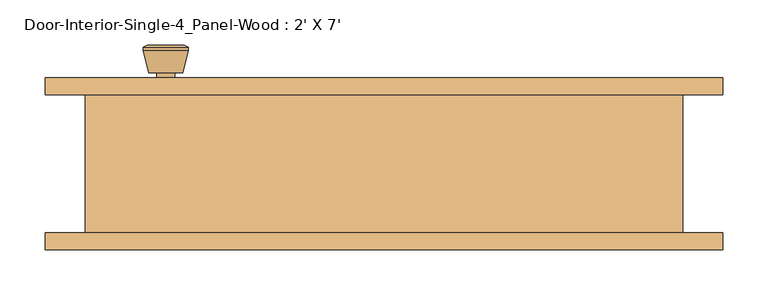
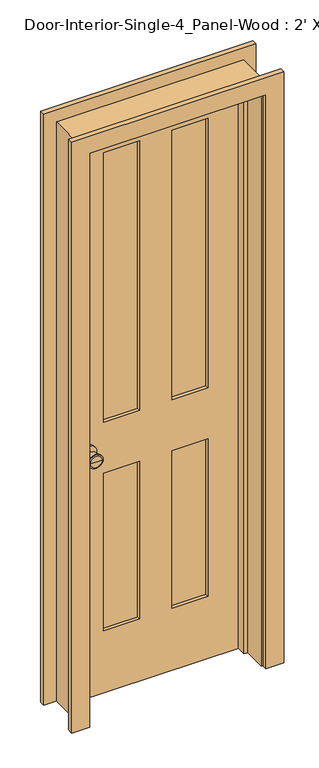
"""IFC4 building model written with IfcOpenShell, lengths in millimetres: door geometry, Door-Interior-Single-4_Panel-Wood : 2' X 7'."""

from ifc_helpers import new_model, si_unit, point, frame, frame_2d, origin, place, context, project, spatial, polyline, circle_curve, trimmed, segment, composite_curve, outline, extrude, faceted_brep, source, transform, mapped, element, save
from ifc_brep_helpers import plane_surface, cylinder_surface, revolved_surface, advanced_brep


def door_interior_single_4_panel_wood_2_x_7_099afc9e(model_context):
    return source(origin(), model_context, "Body", "SolidModel", [
        advanced_brep(
        [(-241.3, 32.1, 914.4), (-231.3, 32.1, 914.4), (-251.3, 32.1, 914.4), (-220.8241324, -16.9, 914.4), (-241.3, -16.9, 914.4), (-261.7758676, -16.9, 914.4), (-216.3, -15.0721319, 914.4), (-266.3, -15.0721319, 914.4), (-216.3, -11.6084537, 914.4), (-266.3, -11.6084537, 914.4), (-222.663764, 13.1, 914.4), (-259.936236, 13.1, 914.4), (-231.3, 13.1, 914.4), (-251.3, 13.1, 914.4)],
        [
            (0, 1),
            (1, 2, circle_curve(frame((-241.3, 32.1, 914.4), z_axis=(0.0, 1.0, 0.0), x_axis=(-1.0, 0.0, 0.0)), 10.0)),
            (2, 0),
            (2, 1, circle_curve(frame((-241.3, 32.1, 914.4), z_axis=(0.0, 1.0, 0.0), x_axis=(-1.0, 0.0, 0.0)), 10.0)),
            (3, 4),
            (4, 5),
            (5, 3, circle_curve(frame((-241.3, -16.9, 914.4), z_axis=(0.0, -1.0, 0.0), x_axis=(-1.0, 0.0, 0.0)), 20.4758676)),
            (3, 5, circle_curve(frame((-241.3, -16.9, 914.4), z_axis=(0.0, -1.0, 0.0), x_axis=(-1.0, 0.0, 0.0)), 20.4758676)),
            (6, 3),
            (5, 7),
            (7, 6, circle_curve(frame((-241.3, -15.0721319, 914.4), z_axis=(0.0, -1.0, 0.0), x_axis=(-1.0, 0.0, 0.0)), 25.0)),
            (6, 7, circle_curve(frame((-241.3, -15.0721319, 914.4), z_axis=(0.0, -1.0, 0.0), x_axis=(-1.0, 0.0, 0.0)), 25.0)),
            (8, 6),
            (7, 9),
            (9, 8, circle_curve(frame((-241.3, -11.6084537, 914.4), z_axis=(0.0, -1.0, 0.0), x_axis=(-1.0, 0.0, 0.0)), 25.0)),
            (8, 9, circle_curve(frame((-241.3, -11.6084537, 914.4), z_axis=(0.0, -1.0, 0.0), x_axis=(-1.0, 0.0, 0.0)), 25.0)),
            (10, 8),
            (9, 11),
            (11, 10, circle_curve(frame((-241.3, 13.1, 914.4), z_axis=(0.0, -1.0, 0.0), x_axis=(-1.0, 0.0, 0.0)), 18.636236)),
            (10, 11, circle_curve(frame((-241.3, 13.1, 914.4), z_axis=(0.0, -1.0, 0.0), x_axis=(-1.0, 0.0, 0.0)), 18.636236)),
            (12, 10),
            (11, 13),
            (13, 12, circle_curve(frame((-241.3, 13.1, 914.4), z_axis=(0.0, -1.0, 0.0), x_axis=(-1.0, 0.0, 0.0)), 10.0)),
            (12, 13, circle_curve(frame((-241.3, 13.1, 914.4), z_axis=(0.0, -1.0, 0.0), x_axis=(-1.0, 0.0, 0.0)), 10.0)),
            (1, 12),
            (13, 2),
        ],
        [
            plane_surface(frame((-241.3, 32.1, 914.4), z_axis=(0.0, 1.0, 0.0), x_axis=(-1.0, 0.0, 0.0))),
            plane_surface(frame((-241.3, -16.9, 914.4), z_axis=(0.0, -1.0, 0.0), x_axis=(-1.0, 0.0, 0.0))),
            revolved_surface(polyline([(-261.7758676, -16.9, 914.4), (-266.3, -15.0721319, 914.4)]), (-241.3, 32.1, 914.4), (0.0, 1.0, 0.0)),
            cylinder_surface(frame((-241.3, 32.1, 914.4), z_axis=(0.0, 1.0, 0.0), x_axis=(-1.0, 0.0, 0.0)), 25.0),
            revolved_surface(polyline([(-266.3, -11.6084537, 914.4), (-259.936236, 13.1, 914.4)]), (-241.3, 32.1, 914.4), (0.0, 1.0, 0.0)),
            plane_surface(frame((-241.3, 13.1, 914.4), z_axis=(0.0, 1.0, 0.0), x_axis=(-1.0, 0.0, 0.0))),
            cylinder_surface(frame((-241.3, 32.1, 914.4), z_axis=(0.0, 1.0, 0.0), x_axis=(-1.0, 0.0, 0.0)), 10.0),
        ],
        [
            (0, [[1, 2, 3]]),
            (0, [[-3, 4, -1]]),
            (1, [[5, 6, 7]]),
            (1, [[-6, -5, 8]]),
            (2, [[9, -7, 10, 11]]),
            (2, [[-10, -8, -9, 12]]),
            (3, [[13, -11, 14, 15]]),
            (3, [[-14, -12, -13, 16]]),
            (4, [[17, -15, 18, 19]]),
            (4, [[-18, -16, -17, 20]]),
            (5, [[21, -19, 22, 23]]),
            (5, [[-22, -20, -21, 24]]),
            (6, [[25, -23, 26, -2]]),
            (6, [[-26, -24, -25, -4]]),
        ],
    ),
        extrude(outline(composite_curve([segment(trimmed(circle_curve(frame_2d((914.4, -241.3)), 30.0), [point((914.4, -271.3))], [point((914.4, -211.3))], False, "CARTESIAN"), True, "CONTINUOUS"), segment(trimmed(circle_curve(frame_2d((914.4, -241.3)), 30.0), [point((914.4, -211.3))], [point((914.4, -271.3))], False, "CARTESIAN"), True, "CONTINUOUS")], self_intersect=False)), frame((0.0, 32.1, 0.0), z_axis=(0.0, 1.0, 0.0), x_axis=(0.0, 0.0, 1.0)), (0.0, 0.0, 1.0), 6.0),
        advanced_brep(
        [(-241.3, 79.025, 914.4), (-251.3, 79.025, 914.4), (-231.3, 79.025, 914.4), (-220.8241324, 128.025, 914.4), (-261.7758676, 128.025, 914.4), (-241.3, 128.025, 914.4), (-216.3, 126.1971319, 914.4), (-266.3, 126.1971319, 914.4), (-216.3, 122.7334537, 914.4), (-266.3, 122.7334537, 914.4), (-222.663764, 98.025, 914.4), (-259.936236, 98.025, 914.4), (-231.3, 98.025, 914.4), (-251.3, 98.025, 914.4)],
        [
            (0, 1),
            (1, 2, circle_curve(frame((-241.3, 79.025, 914.4), z_axis=(0.0, -1.0, 0.0), x_axis=(-1.0, 0.0, 0.0)), 10.0)),
            (2, 0),
            (2, 1, circle_curve(frame((-241.3, 79.025, 914.4), z_axis=(0.0, -1.0, 0.0), x_axis=(-1.0, 0.0, 0.0)), 10.0)),
            (3, 4, circle_curve(frame((-241.3, 128.025, 914.4), z_axis=(0.0, 1.0, 0.0), x_axis=(-1.0, 0.0, 0.0)), 20.4758676)),
            (4, 5),
            (5, 3),
            (4, 3, circle_curve(frame((-241.3, 128.025, 914.4), z_axis=(0.0, 1.0, 0.0), x_axis=(-1.0, 0.0, 0.0)), 20.4758676)),
            (6, 7, circle_curve(frame((-241.3, 126.1971319, 914.4), z_axis=(0.0, 1.0, 0.0), x_axis=(-1.0, 0.0, 0.0)), 25.0)),
            (7, 4),
            (3, 6),
            (7, 6, circle_curve(frame((-241.3, 126.1971319, 914.4), z_axis=(0.0, 1.0, 0.0), x_axis=(-1.0, 0.0, 0.0)), 25.0)),
            (8, 9, circle_curve(frame((-241.3, 122.7334537, 914.4), z_axis=(0.0, 1.0, 0.0), x_axis=(-1.0, 0.0, 0.0)), 25.0)),
            (9, 7),
            (6, 8),
            (9, 8, circle_curve(frame((-241.3, 122.7334537, 914.4), z_axis=(0.0, 1.0, 0.0), x_axis=(-1.0, 0.0, 0.0)), 25.0)),
            (10, 11, circle_curve(frame((-241.3, 98.025, 914.4), z_axis=(0.0, 1.0, 0.0), x_axis=(-1.0, 0.0, 0.0)), 18.636236)),
            (11, 9),
            (8, 10),
            (11, 10, circle_curve(frame((-241.3, 98.025, 914.4), z_axis=(0.0, 1.0, 0.0), x_axis=(-1.0, 0.0, 0.0)), 18.636236)),
            (12, 13, circle_curve(frame((-241.3, 98.025, 914.4), z_axis=(0.0, 1.0, 0.0), x_axis=(-1.0, 0.0, 0.0)), 10.0)),
            (13, 11),
            (10, 12),
            (13, 12, circle_curve(frame((-241.3, 98.025, 914.4), z_axis=(0.0, 1.0, 0.0), x_axis=(-1.0, 0.0, 0.0)), 10.0)),
            (1, 13),
            (12, 2),
        ],
        [
            plane_surface(frame((-241.3, 79.025, 914.4), z_axis=(0.0, -1.0, 0.0), x_axis=(-1.0, 0.0, 0.0))),
            plane_surface(frame((-241.3, 128.025, 914.4), z_axis=(0.0, 1.0, 0.0), x_axis=(-1.0, 0.0, 0.0))),
            revolved_surface(polyline([(-261.7758676, 128.025, 914.4), (-266.3, 126.1971319, 914.4)]), (-241.3, 79.025, 914.4), (0.0, -1.0, 0.0)),
            cylinder_surface(frame((-241.3, 79.025, 914.4), z_axis=(0.0, -1.0, 0.0), x_axis=(-1.0, 0.0, 0.0)), 25.0),
            revolved_surface(polyline([(-266.3, 122.7334537, 914.4), (-259.936236, 98.025, 914.4)]), (-241.3, 79.025, 914.4), (0.0, -1.0, 0.0)),
            plane_surface(frame((-241.3, 98.025, 914.4), z_axis=(0.0, -1.0, 0.0), x_axis=(-1.0, 0.0, 0.0))),
            cylinder_surface(frame((-241.3, 79.025, 914.4), z_axis=(0.0, -1.0, 0.0), x_axis=(-1.0, 0.0, 0.0)), 10.0),
        ],
        [
            (0, [[1, 2, 3]]),
            (0, [[-3, 4, -1]]),
            (1, [[5, 6, 7]]),
            (1, [[8, -7, -6]]),
            (2, [[9, 10, -5, 11]]),
            (2, [[12, -11, -8, -10]]),
            (3, [[13, 14, -9, 15]]),
            (3, [[16, -15, -12, -14]]),
            (4, [[17, 18, -13, 19]]),
            (4, [[20, -19, -16, -18]]),
            (5, [[21, 22, -17, 23]]),
            (5, [[24, -23, -20, -22]]),
            (6, [[-2, 25, -21, 26]]),
            (6, [[-4, -26, -24, -25]]),
        ],
    ),
        extrude(outline(composite_curve([segment(trimmed(circle_curve(frame_2d((914.4, -241.3)), 30.0), [point((914.4, -271.3))], [point((914.4, -211.3))], False, "CARTESIAN"), True, "CONTINUOUS"), segment(trimmed(circle_curve(frame_2d((914.4, -241.3)), 30.0), [point((914.4, -211.3))], [point((914.4, -271.3))], False, "CARTESIAN"), True, "CONTINUOUS")], self_intersect=False)), frame((0.0, 73.025, 0.0), z_axis=(0.0, 1.0, 0.0), x_axis=(0.0, 0.0, 1.0)), (0.0, 0.0, 1.0), 6.0),
        faceted_brep([(330.2, 73.025, 0.0), (330.2, -79.375, 0.0), (304.8, -79.375, 0.0), (304.8, 3.175, 0.0), (292.1, 3.175, 0.0), (292.1, 38.1, 0.0), (304.8, 38.1, 0.0), (304.8, 73.025, 0.0), (330.2, 73.025, 2159.0), (330.2, -79.375, 2159.0), (-330.2, -79.375, 2159.0), (-330.2, -79.375, 0.0), (-304.8, -79.375, 0.0), (-304.8, -79.375, 2133.6), (304.8, -79.375, 2133.6), (304.8, 3.175, 2133.6), (-304.8, 3.175, 2133.6), (-304.8, 3.175, 0.0), (-292.1, 3.175, 0.0), (-292.1, 3.175, 2120.9), (292.1, 3.175, 2120.9), (292.1, 38.1, 2120.9), (-292.1, 38.1, 2120.9), (-292.1, 38.1, 0.0), (-304.8, 38.1, 0.0), (-304.8, 38.1, 2133.6), (304.8, 38.1, 2133.6), (304.8, 73.025, 2133.6), (-304.8, 73.025, 2133.6), (-304.8, 73.025, 0.0), (-330.2, 73.025, 0.0), (-330.2, 73.025, 2159.0)], [[[0, 1, 2, 3, 4, 5, 6, 7]], [[1, 0, 8, 9]], [[2, 1, 9, 10, 11, 12, 13, 14]], [[3, 2, 14, 15]], [[4, 3, 15, 16, 17, 18, 19, 20]], [[5, 4, 20, 21]], [[6, 5, 21, 22, 23, 24, 25, 26]], [[7, 6, 26, 27]], [[0, 7, 27, 28, 29, 30, 31, 8]], [[9, 8, 31, 10]], [[15, 14, 13, 16]], [[21, 20, 19, 22]], [[27, 26, 25, 28]], [[30, 29, 24, 23, 18, 17, 12, 11]], [[10, 31, 30, 11]], [[16, 13, 12, 17]], [[22, 19, 18, 23]], [[28, 25, 24, 29]]]),
        extrude(outline(polyline([(2133.6, -304.8), (0.0, -304.8), (0.0, 304.8), (2133.6, 304.8), (2133.6, -304.8)]), holes=[polyline([(2014.5375, 57.15), (2014.5375, 184.15), (1009.65, 184.15), (1009.65, 57.15), (2014.5375, 57.15)]), polyline([(1009.65, -57.15), (1009.65, -184.15), (2014.5375, -184.15), (2014.5375, -57.15), (1009.65, -57.15)]), polyline([(819.15, 57.15), (819.15, 184.15), (231.775, 184.15), (231.775, 57.15), (819.15, 57.15)]), polyline([(231.775, -57.15), (231.775, -184.15), (819.15, -184.15), (819.15, -57.15), (231.775, -57.15)])]), frame((0.0, 38.1, 0.0), z_axis=(0.0, 1.0, 0.0), x_axis=(0.0, 0.0, 1.0)), (0.0, 0.0, 1.0), 34.925),
        extrude(outline(polyline([(184.15, 49.7416667), (57.15, 49.7416667), (57.15, 61.3833333), (184.15, 61.3833333), (184.15, 49.7416667)])), frame((0.0, 0.0, 1009.65), z_axis=(0.0, 0.0, 1.0), x_axis=(1.0, 0.0, 0.0)), (0.0, 0.0, 1.0), 1004.8875),
        extrude(outline(polyline([(-57.15, 49.7416667), (-184.15, 49.7416667), (-184.15, 61.3833333), (-57.15, 61.3833333), (-57.15, 49.7416667)])), frame((0.0, 0.0, 1009.65), z_axis=(0.0, 0.0, 1.0), x_axis=(1.0, 0.0, 0.0)), (0.0, 0.0, 1.0), 1004.8875),
        extrude(outline(polyline([(184.15, 49.7416667), (57.15, 49.7416667), (57.15, 61.3833333), (184.15, 61.3833333), (184.15, 49.7416667)])), frame((0.0, 0.0, 231.775), z_axis=(0.0, 0.0, 1.0), x_axis=(1.0, 0.0, 0.0)), (0.0, 0.0, 1.0), 587.375),
        extrude(outline(polyline([(-57.15, 49.7416667), (-184.15, 49.7416667), (-184.15, 61.3833333), (-57.15, 61.3833333), (-57.15, 49.7416667)])), frame((0.0, 0.0, 231.775), z_axis=(0.0, 0.0, 1.0), x_axis=(1.0, 0.0, 0.0)), (0.0, 0.0, 1.0), 587.375),
        extrude(outline(polyline([(0.0, 311.15), (0.0, 374.65), (2203.45, 374.65), (2203.45, -374.65), (0.0, -374.65), (0.0, -311.15), (2139.95, -311.15), (2139.95, 311.15), (0.0, 311.15)])), frame((0.0, 73.025, 0.0), z_axis=(0.0, 1.0, 0.0), x_axis=(0.0, 0.0, 1.0)), (0.0, 0.0, 1.0), 19.05),
        extrude(outline(polyline([(0.0, 311.15), (0.0, 374.65), (2203.45, 374.65), (2203.45, -374.65), (0.0, -374.65), (0.0, -311.15), (2139.95, -311.15), (2139.95, 311.15), (0.0, 311.15)])), frame((0.0, -98.425, 0.0), z_axis=(0.0, 1.0, 0.0), x_axis=(0.0, 0.0, 1.0)), (0.0, 0.0, 1.0), 19.05),
    ])


if __name__ == "__main__":
    model = new_model("IFC4")
    model_context = context("Model", 3, world=origin())
    ifc_project = project(units=[si_unit("LENGTHUNIT", "METRE", prefix="MILLI")], contexts=[model_context])
    site = spatial("IfcSite", under=ifc_project)
    building = spatial("IfcBuilding", under=site)
    placement = place(None, origin())
    door_interior_single_4_panel_wood_2_x_7_shape = door_interior_single_4_panel_wood_2_x_7_099afc9e(model_context)
    element("IfcDoor", 1, ObjectType="Door-Interior-Single-4_Panel-Wood : 2' X 7'", at=placement, inside=building, context=model_context, shape_type="MappedRepresentation", body=[
        mapped(door_interior_single_4_panel_wood_2_x_7_shape, transform((0.0, 0.0, 0.0), x_axis=(1.0, 0.0, 0.0), y_axis=(0.0, 1.0, 0.0), z_axis=(0.0, 0.0, 1.0))),
    ])
    save(model, "model.ifc")

# Revit data of these elements
# Type "Door-Interior-Single-4_Panel-Wood : 2' X 7'"
#   Type Mark = "17"
#   Assembly Code = "C1020300"
#   Analytic Construction = "Wooden"
#   Top Rail = 0' - 4 11/16"
#   Thickness = 0' - 1 3/8"
#   Thermal Resistance (R) = 2.5876 (h·ft²·°F)/BTU
#   Swing Angle [instance default] = 90.00°
#   Stiles = 0' - 4 3/4"
#   Rough Width = 2' - 2"
#   Rough Height = 7' - 1"
#   Mullion = 0' - 4 1/2"
#   Lock Rail = 0' - 7 1/2"
#   Height = 7' - 0"
#   Width = 2' - 0"
#   Heat Transfer Coefficient (U) = 0.3865 BTU/(h·ft²·°F)
#   Bottom Rail = 0' - 9 1/8"
#   Trim Material = Cherry
#   Panel Material = Cherry
#   Frame Material = Cherry
#   Door Handle Material = Aluminum
#   Visual Light Transmittance = 0
#   Solar Heat Gain Coefficient = 0
#   Wall Closure = (empty or 0)
#   Function = (empty or 0)
# Element 1 (IfcDoor, "Door-Interior-Single-4_Panel-Wood : 2' X 7'")
#   Materials on its faces: "Cherry", "Aluminum"
# Materials
#   "Cherry": class "Wood", colour RGB 226 177 128, transparency 0, Description = "Prunus Serotina", Cost = 0
#   "Aluminum": class "Metal", colour RGB 247 247 247, transparency 0, Description = "Aluminum 6061", Cost = 0
